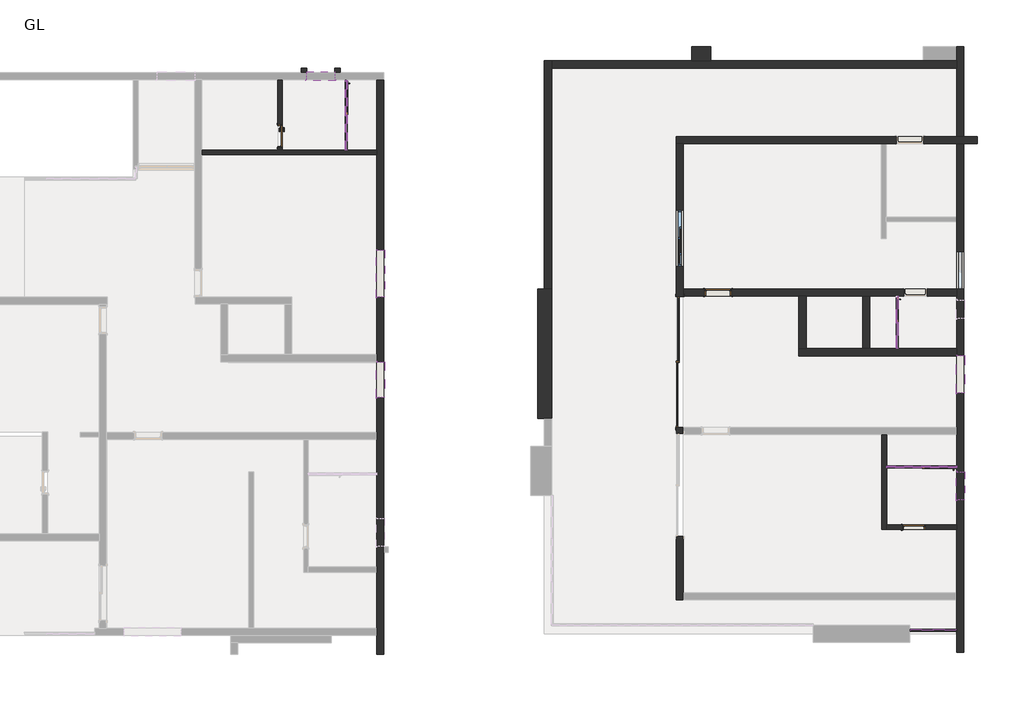
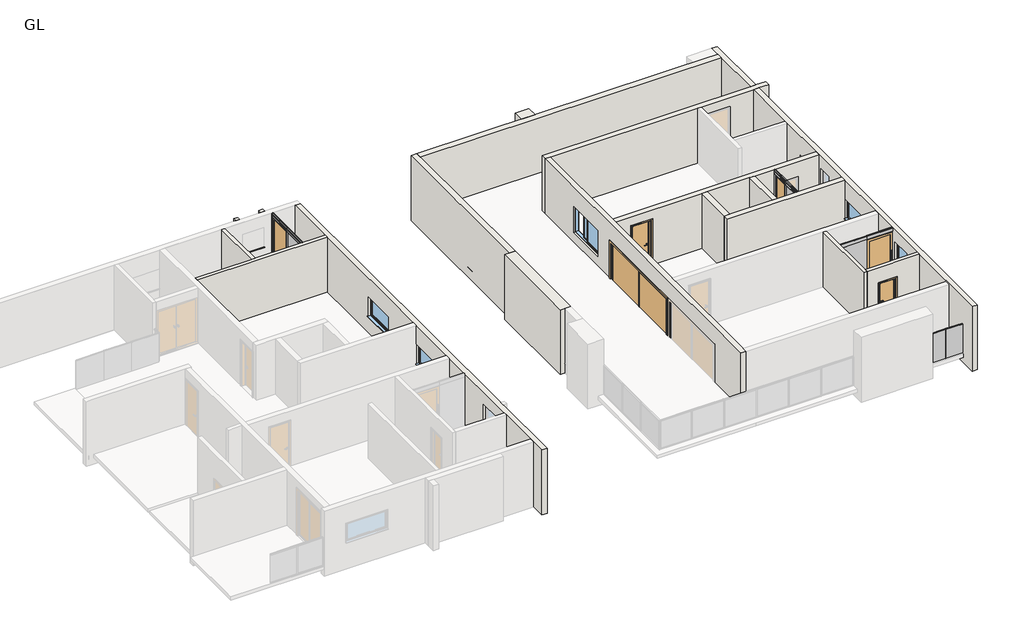
# One storey, part 4 of 6: 41 members, 18 walls, 11 plates, 7 doors, 6 windows.
"""IFC4 building model written with IfcOpenShell, lengths in millimetres."""

from ifc_helpers import new_model, si_unit, frame, origin, origin_with_axes, place, context, project, spatial, polyline, outline, extrude, faceted_brep, transform, mapped, element, save
from components import door_14_4c4e9c4f, door_b7cddb0a, doors_intsgl_2_5_fba66aca, doors_sgl_glass_1_glass_panel_12mm_thickness_3d57b09a, doors_sgl_glass_1_glass_panel_12mm_thickness_ae7dd786, doors_sgl_glass_1_glass_panel_12mm_thickness_d76e1df9, rectangular_mullion_30mm_square_7ad516a4, rectangular_mullion_30mm_square_4b249e81, rectangular_mullion_30mm_square_9902f449, rectangular_mullion_30mm_square_eec092c3, rectangular_mullion_30mm_square_9325025b, rectangular_mullion_30mm_square_b25d63a0, rectangular_mullion_30mm_square_e994106c, rectangular_mullion_30mm_square_28ebc8b3, rectangular_mullion_30mm_square_b4ecd99e, rectangular_mullion_30mm_square_e2360202, rectangular_mullion_30mm_square_9211323b, rectangular_mullion_30mm_square_b0565101, rectangular_mullion_30mm_square_fdabec93, system_panel_glazed_78f80fad, system_panel_glazed_cac99656, system_panel_glazed_6c2d91e7, system_panel_glazed_d770e50e, system_panel_glazed_325d72d1, system_panel_glazed_2af15f36, system_panel_glazed_747750e0, parametric_operable_sliding_window_6387_6_8dd7d652, windows_sgl_plain_3_28d0678b, window_6a333e19, windows_sgl_plain_4_aaf4c78a, windows_sgl_plain_5_79f17ecf

model = new_model("IFC4")

# Units and contexts
model_context = context("Model", 3, world=origin())
ifc_project = project(units=[si_unit("LENGTHUNIT", "METRE", prefix="MILLI")], contexts=[model_context])

# Site, building, storey
site = spatial("IfcSite", under=ifc_project)
building = spatial("IfcBuilding", under=site)
storey = spatial("IfcBuildingStorey", under=building, Name="GL", Elevation=0.0)

# Doors
placement = place(None, origin())
door_14_shape = door_14_4c4e9c4f(model_context)
element("IfcDoor", 1, ObjectType="14'", at=placement, inside=storey, context=model_context, shape_type="MappedRepresentation", body=[
    mapped(door_14_shape, transform((-5795.6337573, 17869.1220058, 0.0), x_axis=(0.0, 1.0, 0.0), y_axis=(-1.0, 0.0, 0.0), z_axis=(0.0, 0.0, 1.0))),
])
door_shape = door_b7cddb0a(model_context)
element("IfcDoor", 2, ObjectType="Doors_IntSgl : 2'11\"", at=placement, inside=storey, context=model_context, shape_type="MappedRepresentation", body=[
    mapped(door_shape, transform((-4678.0337573, 20128.7664182, 449.9570313), x_axis=(-1.0, 0.0, 0.0), y_axis=(0.0, -1.0, 0.0), z_axis=(0.0, 0.0, 1.0))),
])
doors_intsgl_2_5_shape = doors_intsgl_2_5_fba66aca(model_context)
element("IfcDoor", 3, ObjectType="Doors_IntSgl : 2.5'", at=placement, inside=storey, context=model_context, shape_type="MappedRepresentation", body=[
    mapped(doors_intsgl_2_5_shape, transform((-18933.3266085, 25228.098106, 0.0), x_axis=(0.0, -1.0, 0.0), y_axis=(1.0, 0.0, 0.0), z_axis=(0.0, 0.0, 1.0))),
])
element("IfcDoor", 4, ObjectType="Doors_IntSgl : 2.5'", at=placement, inside=storey, context=model_context, shape_type="MappedRepresentation", body=[
    mapped(doors_intsgl_2_5_shape, transform((1696.7626485, 12484.3220058, 449.9570313), x_axis=(1.0, 0.0, 0.0), y_axis=(0.0, 1.0, 0.0), z_axis=(0.0, 0.0, 1.0))),
])
doors_sgl_glass_1_glass_panel_12mm_thickness_shape = doors_sgl_glass_1_glass_panel_12mm_thickness_3d57b09a(model_context)
element("IfcDoor", 5, ObjectType="Doors_Sgl_Glass_1 : Glass_Panel-12mm_Thickness", at=placement, inside=storey, context=model_context, shape_type="MappedRepresentation", body=[
    mapped(doors_sgl_glass_1_glass_panel_12mm_thickness_shape, transform((-16799.7266085, 26469.8075628, 479.9570313), x_axis=(0.0, -1.0, 0.0), y_axis=(1.0, 0.0, 0.0), z_axis=(0.0, 0.0, 1.0))),
])
doors_sgl_glass_1_glass_panel_12mm_thickness_2_shape = doors_sgl_glass_1_glass_panel_12mm_thickness_ae7dd786(model_context)
element("IfcDoor", 6, ObjectType="Doors_Sgl_Glass_1 : Glass_Panel-12mm_Thickness", at=placement, inside=storey, context=model_context, shape_type="MappedRepresentation", body=[
    mapped(doors_sgl_glass_1_glass_panel_12mm_thickness_2_shape, transform((2515.5764369, 14465.5220058, 479.9570313), x_axis=(-1.0, 0.0, 0.0), y_axis=(0.0, -1.0, 0.0), z_axis=(0.0, 0.0, 1.0))),
])
doors_sgl_glass_1_glass_panel_12mm_thickness_3_shape = doors_sgl_glass_1_glass_panel_12mm_thickness_d76e1df9(model_context)
element("IfcDoor", 7, ObjectType="Doors_Sgl_Glass_1 : Glass_Panel-12mm_Thickness", at=placement, inside=storey, context=model_context, shape_type="MappedRepresentation", body=[
    mapped(doors_sgl_glass_1_glass_panel_12mm_thickness_3_shape, transform((1132.6976997, 19578.0085204, 479.9570313), x_axis=(0.0, -1.0, 0.0), y_axis=(1.0, 0.0, 0.0), z_axis=(0.0, 0.0, 1.0))),
])

# Members
rectangular_mullion_30mm_square_shape = rectangular_mullion_30mm_square_7ad516a4(model_context)
element("IfcMember", 8, ObjectType="Rectangular Mullion : 30mm_Square", at=placement, inside=storey, context=model_context, shape_type="MappedRepresentation", body=[
    mapped(rectangular_mullion_30mm_square_shape, transform((2330.3942124, 9140.7448884, 449.9570313), x_axis=(-1.0, 0.0, 0.0), y_axis=(0.0, 1.0, 0.0), z_axis=(0.0, 0.0, -1.0))),
])
rectangular_mullion_30mm_square_2_shape = rectangular_mullion_30mm_square_4b249e81(model_context)
element("IfcMember", 9, ObjectType="Rectangular Mullion : 30mm_Square", at=placement, inside=storey, context=model_context, shape_type="MappedRepresentation", body=[
    mapped(rectangular_mullion_30mm_square_2_shape, transform((3094.8476997, 9140.7448884, 1780.8), x_axis=(1.0, 0.0, 0.0), y_axis=(0.0, 1.0, 0.0), z_axis=(0.0, 0.0, 1.0))),
])
element("IfcMember", 10, ObjectType="Rectangular Mullion : 30mm_Square", at=placement, inside=storey, context=model_context, shape_type="MappedRepresentation", body=[
    mapped(rectangular_mullion_30mm_square_2_shape, transform((1565.9407251, 9140.7448884, 449.9570313), x_axis=(-1.0, 0.0, 0.0), y_axis=(0.0, 1.0, 0.0), z_axis=(0.0, 0.0, -1.0))),
])
rectangular_mullion_30mm_square_3_shape = rectangular_mullion_30mm_square_9902f449(model_context)
element("IfcMember", 11, ObjectType="Rectangular Mullion : 30mm_Square", at=placement, inside=storey, context=model_context, shape_type="MappedRepresentation", body=[
    mapped(rectangular_mullion_30mm_square_3_shape, transform((1595.9407251, 9140.7448884, 1780.8), x_axis=(0.0, 0.0, 1.0), y_axis=(0.0, 1.0, 0.0), z_axis=(-1.0, 0.0, 0.0))),
])
element("IfcMember", 12, ObjectType="Rectangular Mullion : 30mm_Square", at=placement, inside=storey, context=model_context, shape_type="MappedRepresentation", body=[
    mapped(rectangular_mullion_30mm_square_3_shape, transform((2345.3942124, 9140.7448884, 1780.8), x_axis=(0.0, 0.0, 1.0), y_axis=(0.0, 1.0, 0.0), z_axis=(-1.0, 0.0, 0.0))),
])
element("IfcMember", 13, ObjectType="Rectangular Mullion : 30mm_Square", at=placement, inside=storey, context=model_context, shape_type="MappedRepresentation", body=[
    mapped(rectangular_mullion_30mm_square_3_shape, transform((3064.8476997, 9140.7448884, 449.9570313), x_axis=(0.0, 0.0, -1.0), y_axis=(0.0, 1.0, 0.0), z_axis=(1.0, 0.0, 0.0))),
])
element("IfcMember", 14, ObjectType="Rectangular Mullion : 30mm_Square", at=placement, inside=storey, context=model_context, shape_type="MappedRepresentation", body=[
    mapped(rectangular_mullion_30mm_square_3_shape, transform((2315.3942124, 9140.7448884, 449.9570313), x_axis=(0.0, 0.0, -1.0), y_axis=(0.0, 1.0, 0.0), z_axis=(1.0, 0.0, 0.0))),
])
rectangular_mullion_30mm_square_4_shape = rectangular_mullion_30mm_square_eec092c3(model_context)
element("IfcMember", 15, ObjectType="Rectangular Mullion : 30mm_Square", at=placement, inside=storey, context=model_context, shape_type="MappedRepresentation", body=[
    mapped(rectangular_mullion_30mm_square_4_shape, transform((-16799.7266085, 24800.898106, 3000.0), x_axis=(0.0, 0.0, 1.0), y_axis=(-1.0, 0.0, 0.0), z_axis=(0.0, -1.0, 0.0))),
])
element("IfcMember", 16, ObjectType="Rectangular Mullion : 30mm_Square", at=placement, inside=storey, context=model_context, shape_type="MappedRepresentation", body=[
    mapped(rectangular_mullion_30mm_square_4_shape, transform((-16799.7266085, 25923.5044105, 3000.0), x_axis=(0.0, 0.0, 1.0), y_axis=(-1.0, 0.0, 0.0), z_axis=(0.0, -1.0, 0.0))),
])
element("IfcMember", 17, ObjectType="Rectangular Mullion : 30mm_Square", at=placement, inside=storey, context=model_context, shape_type="MappedRepresentation", body=[
    mapped(rectangular_mullion_30mm_square_4_shape, transform((-16799.7266085, 27016.1107151, 449.9570313), x_axis=(0.0, 0.0, -1.0), y_axis=(-1.0, 0.0, 0.0), z_axis=(0.0, 1.0, 0.0))),
])
element("IfcMember", 18, ObjectType="Rectangular Mullion : 30mm_Square", at=placement, inside=storey, context=model_context, shape_type="MappedRepresentation", body=[
    mapped(rectangular_mullion_30mm_square_4_shape, transform((-16799.7266085, 25893.5044105, 449.9570313), x_axis=(0.0, 0.0, -1.0), y_axis=(-1.0, 0.0, 0.0), z_axis=(0.0, 1.0, 0.0))),
])
rectangular_mullion_30mm_square_5_shape = rectangular_mullion_30mm_square_9325025b(model_context)
element("IfcMember", 19, ObjectType="Rectangular Mullion : 30mm_Square", at=placement, inside=storey, context=model_context, shape_type="MappedRepresentation", body=[
    mapped(rectangular_mullion_30mm_square_5_shape, transform((-16799.7266085, 25908.5044105, 449.9570313), x_axis=(0.0, -1.0, 0.0), y_axis=(-1.0, 0.0, 0.0), z_axis=(0.0, 0.0, -1.0))),
])
element("IfcMember", 20, ObjectType="Rectangular Mullion : 30mm_Square", at=placement, inside=storey, context=model_context, shape_type="MappedRepresentation", body=[
    mapped(rectangular_mullion_30mm_square_5_shape, transform((1951.3051741, 14465.5220058, 449.9570313), x_axis=(-1.0, 0.0, 0.0), y_axis=(0.0, 1.0, 0.0), z_axis=(0.0, 0.0, -1.0))),
])
element("IfcMember", 21, ObjectType="Rectangular Mullion : 30mm_Square", at=placement, inside=storey, context=model_context, shape_type="MappedRepresentation", body=[
    mapped(rectangular_mullion_30mm_square_5_shape, transform((1132.6976997, 19156.5506226, 449.9570313), x_axis=(0.0, -1.0, 0.0), y_axis=(-1.0, 0.0, 0.0), z_axis=(0.0, 0.0, -1.0))),
])
rectangular_mullion_30mm_square_6_shape = rectangular_mullion_30mm_square_b25d63a0(model_context)
element("IfcMember", 22, ObjectType="Rectangular Mullion : 30mm_Square", at=placement, inside=storey, context=model_context, shape_type="MappedRepresentation", body=[
    mapped(rectangular_mullion_30mm_square_6_shape, transform((-16799.7266085, 25923.5044105, 2849.9570312), x_axis=(0.0, 0.0, 1.0), y_axis=(-1.0, 0.0, 0.0), z_axis=(0.0, -1.0, 0.0))),
])
element("IfcMember", 23, ObjectType="Rectangular Mullion : 30mm_Square", at=placement, inside=storey, context=model_context, shape_type="MappedRepresentation", body=[
    mapped(rectangular_mullion_30mm_square_6_shape, transform((-16799.7266085, 24800.898106, 2849.9570312), x_axis=(0.0, 0.0, 1.0), y_axis=(-1.0, 0.0, 0.0), z_axis=(0.0, -1.0, 0.0))),
])
rectangular_mullion_30mm_square_7_shape = rectangular_mullion_30mm_square_e994106c(model_context)
element("IfcMember", 24, ObjectType="Rectangular Mullion : 30mm_Square", at=placement, inside=storey, context=model_context, shape_type="MappedRepresentation", body=[
    mapped(rectangular_mullion_30mm_square_7_shape, transform((-16799.7266085, 25908.5044105, 2849.9570312), x_axis=(0.0, -1.0, 0.0), y_axis=(-1.0, 0.0, 0.0), z_axis=(0.0, 0.0, -1.0))),
])
element("IfcMember", 25, ObjectType="Rectangular Mullion : 30mm_Square", at=placement, inside=storey, context=model_context, shape_type="MappedRepresentation", body=[
    mapped(rectangular_mullion_30mm_square_7_shape, transform((1951.3051741, 14465.5220058, 2849.9570312), x_axis=(-1.0, 0.0, 0.0), y_axis=(0.0, 1.0, 0.0), z_axis=(0.0, 0.0, -1.0))),
])
element("IfcMember", 26, ObjectType="Rectangular Mullion : 30mm_Square", at=placement, inside=storey, context=model_context, shape_type="MappedRepresentation", body=[
    mapped(rectangular_mullion_30mm_square_7_shape, transform((1132.6976997, 19156.5506226, 2849.9570312), x_axis=(0.0, -1.0, 0.0), y_axis=(-1.0, 0.0, 0.0), z_axis=(0.0, 0.0, -1.0))),
])
rectangular_mullion_30mm_square_8_shape = rectangular_mullion_30mm_square_28ebc8b3(model_context)
element("IfcMember", 27, ObjectType="Rectangular Mullion : 30mm_Square", at=placement, inside=storey, context=model_context, shape_type="MappedRepresentation", body=[
    mapped(rectangular_mullion_30mm_square_8_shape, transform((-16799.7266085, 27046.1107151, 3000.0), x_axis=(0.0, 1.0, 0.0), y_axis=(-1.0, 0.0, 0.0), z_axis=(0.0, 0.0, 1.0))),
])
element("IfcMember", 28, ObjectType="Rectangular Mullion : 30mm_Square", at=placement, inside=storey, context=model_context, shape_type="MappedRepresentation", body=[
    mapped(rectangular_mullion_30mm_square_8_shape, transform((3094.8476997, 14465.5220058, 3000.0), x_axis=(1.0, 0.0, 0.0), y_axis=(0.0, 1.0, 0.0), z_axis=(0.0, 0.0, 1.0))),
])
rectangular_mullion_30mm_square_9_shape = rectangular_mullion_30mm_square_b4ecd99e(model_context)
element("IfcMember", 29, ObjectType="Rectangular Mullion : 30mm_Square", at=placement, inside=storey, context=model_context, shape_type="MappedRepresentation", body=[
    mapped(rectangular_mullion_30mm_square_9_shape, transform((-16799.7266085, 24770.898106, 449.9570313), x_axis=(0.0, -1.0, 0.0), y_axis=(-1.0, 0.0, 0.0), z_axis=(0.0, 0.0, -1.0))),
])
element("IfcMember", 30, ObjectType="Rectangular Mullion : 30mm_Square", at=placement, inside=storey, context=model_context, shape_type="MappedRepresentation", body=[
    mapped(rectangular_mullion_30mm_square_9_shape, transform((807.7626485, 14465.5220058, 449.9570313), x_axis=(-1.0, 0.0, 0.0), y_axis=(0.0, 1.0, 0.0), z_axis=(0.0, 0.0, -1.0))),
])
element("IfcMember", 31, ObjectType="Rectangular Mullion : 30mm_Square", at=placement, inside=storey, context=model_context, shape_type="MappedRepresentation", body=[
    mapped(rectangular_mullion_30mm_square_9_shape, transform((1132.6976997, 18298.634827, 449.9570313), x_axis=(0.0, -1.0, 0.0), y_axis=(-1.0, 0.0, 0.0), z_axis=(0.0, 0.0, -1.0))),
])
element("IfcMember", 32, ObjectType="Rectangular Mullion : 30mm_Square", at=placement, inside=storey, context=model_context, shape_type="MappedRepresentation", body=[
    mapped(rectangular_mullion_30mm_square_8_shape, transform((-16799.7266085, 24770.898106, 2849.9570312), x_axis=(0.0, -1.0, 0.0), y_axis=(-1.0, 0.0, 0.0), z_axis=(0.0, 0.0, -1.0))),
])
element("IfcMember", 33, ObjectType="Rectangular Mullion : 30mm_Square", at=placement, inside=storey, context=model_context, shape_type="MappedRepresentation", body=[
    mapped(rectangular_mullion_30mm_square_8_shape, transform((807.7626485, 14465.5220058, 2849.9570312), x_axis=(-1.0, 0.0, 0.0), y_axis=(0.0, 1.0, 0.0), z_axis=(0.0, 0.0, -1.0))),
])
element("IfcMember", 34, ObjectType="Rectangular Mullion : 30mm_Square", at=placement, inside=storey, context=model_context, shape_type="MappedRepresentation", body=[
    mapped(rectangular_mullion_30mm_square_8_shape, transform((1132.6976997, 18298.634827, 2849.9570312), x_axis=(0.0, -1.0, 0.0), y_axis=(-1.0, 0.0, 0.0), z_axis=(0.0, 0.0, -1.0))),
])
element("IfcMember", 35, ObjectType="Rectangular Mullion : 30mm_Square", at=placement, inside=storey, context=model_context, shape_type="MappedRepresentation", body=[
    mapped(rectangular_mullion_30mm_square_9_shape, transform((-16799.7266085, 27046.1107151, 2849.9570312), x_axis=(0.0, 1.0, 0.0), y_axis=(-1.0, 0.0, 0.0), z_axis=(0.0, 0.0, 1.0))),
])
element("IfcMember", 36, ObjectType="Rectangular Mullion : 30mm_Square", at=placement, inside=storey, context=model_context, shape_type="MappedRepresentation", body=[
    mapped(rectangular_mullion_30mm_square_9_shape, transform((3094.8476997, 14465.5220058, 2849.9570312), x_axis=(1.0, 0.0, 0.0), y_axis=(0.0, 1.0, 0.0), z_axis=(0.0, 0.0, 1.0))),
])
rectangular_mullion_30mm_square_10_shape = rectangular_mullion_30mm_square_e2360202(model_context)
element("IfcMember", 37, ObjectType="Rectangular Mullion : 30mm_Square", at=placement, inside=storey, context=model_context, shape_type="MappedRepresentation", body=[
    mapped(rectangular_mullion_30mm_square_10_shape, transform((837.7626485, 14465.5220058, 3000.0), x_axis=(0.0, 0.0, 1.0), y_axis=(0.0, 1.0, 0.0), z_axis=(-1.0, 0.0, 0.0))),
])
element("IfcMember", 38, ObjectType="Rectangular Mullion : 30mm_Square", at=placement, inside=storey, context=model_context, shape_type="MappedRepresentation", body=[
    mapped(rectangular_mullion_30mm_square_10_shape, transform((1966.3051741, 14465.5220058, 3000.0), x_axis=(0.0, 0.0, 1.0), y_axis=(0.0, 1.0, 0.0), z_axis=(-1.0, 0.0, 0.0))),
])
element("IfcMember", 39, ObjectType="Rectangular Mullion : 30mm_Square", at=placement, inside=storey, context=model_context, shape_type="MappedRepresentation", body=[
    mapped(rectangular_mullion_30mm_square_10_shape, transform((3064.8476997, 14465.5220058, 449.9570313), x_axis=(0.0, 0.0, -1.0), y_axis=(0.0, 1.0, 0.0), z_axis=(1.0, 0.0, 0.0))),
])
element("IfcMember", 40, ObjectType="Rectangular Mullion : 30mm_Square", at=placement, inside=storey, context=model_context, shape_type="MappedRepresentation", body=[
    mapped(rectangular_mullion_30mm_square_10_shape, transform((1936.3051741, 14465.5220058, 449.9570313), x_axis=(0.0, 0.0, -1.0), y_axis=(0.0, 1.0, 0.0), z_axis=(1.0, 0.0, 0.0))),
])
rectangular_mullion_30mm_square_11_shape = rectangular_mullion_30mm_square_9211323b(model_context)
element("IfcMember", 41, ObjectType="Rectangular Mullion : 30mm_Square", at=placement, inside=storey, context=model_context, shape_type="MappedRepresentation", body=[
    mapped(rectangular_mullion_30mm_square_11_shape, transform((1966.3051741, 14465.5220058, 2849.9570312), x_axis=(0.0, 0.0, 1.0), y_axis=(0.0, 1.0, 0.0), z_axis=(-1.0, 0.0, 0.0))),
])
element("IfcMember", 42, ObjectType="Rectangular Mullion : 30mm_Square", at=placement, inside=storey, context=model_context, shape_type="MappedRepresentation", body=[
    mapped(rectangular_mullion_30mm_square_11_shape, transform((837.7626485, 14465.5220058, 2849.9570312), x_axis=(0.0, 0.0, 1.0), y_axis=(0.0, 1.0, 0.0), z_axis=(-1.0, 0.0, 0.0))),
])
rectangular_mullion_30mm_square_12_shape = rectangular_mullion_30mm_square_b0565101(model_context)
element("IfcMember", 43, ObjectType="Rectangular Mullion : 30mm_Square", at=placement, inside=storey, context=model_context, shape_type="MappedRepresentation", body=[
    mapped(rectangular_mullion_30mm_square_12_shape, transform((1132.6976997, 18328.634827, 3000.0), x_axis=(0.0, 0.0, 1.0), y_axis=(-1.0, 0.0, 0.0), z_axis=(0.0, -1.0, 0.0))),
])
element("IfcMember", 44, ObjectType="Rectangular Mullion : 30mm_Square", at=placement, inside=storey, context=model_context, shape_type="MappedRepresentation", body=[
    mapped(rectangular_mullion_30mm_square_12_shape, transform((1132.6976997, 19171.5506226, 3000.0), x_axis=(0.0, 0.0, 1.0), y_axis=(-1.0, 0.0, 0.0), z_axis=(0.0, -1.0, 0.0))),
])
element("IfcMember", 45, ObjectType="Rectangular Mullion : 30mm_Square", at=placement, inside=storey, context=model_context, shape_type="MappedRepresentation", body=[
    mapped(rectangular_mullion_30mm_square_12_shape, transform((1132.6976997, 19984.4664182, 449.9570313), x_axis=(0.0, 0.0, -1.0), y_axis=(-1.0, 0.0, 0.0), z_axis=(0.0, 1.0, 0.0))),
])
element("IfcMember", 46, ObjectType="Rectangular Mullion : 30mm_Square", at=placement, inside=storey, context=model_context, shape_type="MappedRepresentation", body=[
    mapped(rectangular_mullion_30mm_square_12_shape, transform((1132.6976997, 19141.5506226, 449.9570313), x_axis=(0.0, 0.0, -1.0), y_axis=(-1.0, 0.0, 0.0), z_axis=(0.0, 1.0, 0.0))),
])
rectangular_mullion_30mm_square_13_shape = rectangular_mullion_30mm_square_fdabec93(model_context)
element("IfcMember", 47, ObjectType="Rectangular Mullion : 30mm_Square", at=placement, inside=storey, context=model_context, shape_type="MappedRepresentation", body=[
    mapped(rectangular_mullion_30mm_square_13_shape, transform((1132.6976997, 19171.5506226, 2849.9570312), x_axis=(0.0, 0.0, 1.0), y_axis=(-1.0, 0.0, 0.0), z_axis=(0.0, -1.0, 0.0))),
])
element("IfcMember", 48, ObjectType="Rectangular Mullion : 30mm_Square", at=placement, inside=storey, context=model_context, shape_type="MappedRepresentation", body=[
    mapped(rectangular_mullion_30mm_square_13_shape, transform((1132.6976997, 18328.634827, 2849.9570312), x_axis=(0.0, 0.0, 1.0), y_axis=(-1.0, 0.0, 0.0), z_axis=(0.0, -1.0, 0.0))),
])

# Plates
system_panel_glazed_shape = system_panel_glazed_78f80fad(model_context)
element("IfcPlate", 49, ObjectType="System Panel : Glazed", at=placement, inside=storey, context=model_context, shape_type="MappedRepresentation", body=[
    mapped(system_panel_glazed_shape, transform((2712.6209561, 9140.7448884, 449.9570313), x_axis=(-1.0, 0.0, 0.0), y_axis=(0.0, -1.0, 0.0), z_axis=(0.0, 0.0, 1.0))),
])
element("IfcPlate", 50, ObjectType="System Panel : Glazed", at=placement, inside=storey, context=model_context, shape_type="MappedRepresentation", body=[
    mapped(system_panel_glazed_shape, transform((1948.1674688, 9140.7448884, 449.9570313), x_axis=(-1.0, 0.0, 0.0), y_axis=(0.0, -1.0, 0.0), z_axis=(0.0, 0.0, 1.0))),
])
system_panel_glazed_2_shape = system_panel_glazed_cac99656(model_context)
element("IfcPlate", 51, ObjectType="System Panel : Glazed", at=placement, inside=storey, context=model_context, shape_type="MappedRepresentation", body=[
    mapped(system_panel_glazed_2_shape, transform((-16799.7266085, 25339.7012583, 449.9570313), x_axis=(0.0, -1.0, 0.0), y_axis=(1.0, 0.0, 0.0), z_axis=(0.0, 0.0, 1.0))),
])
system_panel_glazed_3_shape = system_panel_glazed_6c2d91e7(model_context)
element("IfcPlate", 52, ObjectType="System Panel : Glazed", at=placement, inside=storey, context=model_context, shape_type="MappedRepresentation", body=[
    mapped(system_panel_glazed_3_shape, transform((-16799.7266085, 26477.3075628, 2849.9570312), x_axis=(0.0, -1.0, 0.0), y_axis=(1.0, 0.0, 0.0), z_axis=(0.0, 0.0, 1.0))),
])
element("IfcPlate", 53, ObjectType="System Panel : Glazed", at=placement, inside=storey, context=model_context, shape_type="MappedRepresentation", body=[
    mapped(system_panel_glazed_3_shape, transform((-16799.7266085, 25339.7012583, 2849.9570312), x_axis=(0.0, -1.0, 0.0), y_axis=(1.0, 0.0, 0.0), z_axis=(0.0, 0.0, 1.0))),
])
system_panel_glazed_4_shape = system_panel_glazed_d770e50e(model_context)
element("IfcPlate", 54, ObjectType="System Panel : Glazed", at=placement, inside=storey, context=model_context, shape_type="MappedRepresentation", body=[
    mapped(system_panel_glazed_4_shape, transform((1379.5339113, 14465.5220058, 449.9570313), x_axis=(-1.0, 0.0, 0.0), y_axis=(0.0, -1.0, 0.0), z_axis=(0.0, 0.0, 1.0))),
])
system_panel_glazed_5_shape = system_panel_glazed_325d72d1(model_context)
element("IfcPlate", 55, ObjectType="System Panel : Glazed", at=placement, inside=storey, context=model_context, shape_type="MappedRepresentation", body=[
    mapped(system_panel_glazed_5_shape, transform((2523.0764369, 14465.5220058, 2849.9570312), x_axis=(-1.0, 0.0, 0.0), y_axis=(0.0, -1.0, 0.0), z_axis=(0.0, 0.0, 1.0))),
])
element("IfcPlate", 56, ObjectType="System Panel : Glazed", at=placement, inside=storey, context=model_context, shape_type="MappedRepresentation", body=[
    mapped(system_panel_glazed_5_shape, transform((1379.5339113, 14465.5220058, 2849.9570312), x_axis=(-1.0, 0.0, 0.0), y_axis=(0.0, -1.0, 0.0), z_axis=(0.0, 0.0, 1.0))),
])
system_panel_glazed_6_shape = system_panel_glazed_2af15f36(model_context)
element("IfcPlate", 57, ObjectType="System Panel : Glazed", at=placement, inside=storey, context=model_context, shape_type="MappedRepresentation", body=[
    mapped(system_panel_glazed_6_shape, transform((1132.6976997, 18727.5927248, 449.9570313), x_axis=(0.0, -1.0, 0.0), y_axis=(1.0, 0.0, 0.0), z_axis=(0.0, 0.0, 1.0))),
])
system_panel_glazed_7_shape = system_panel_glazed_747750e0(model_context)
element("IfcPlate", 58, ObjectType="System Panel : Glazed", at=placement, inside=storey, context=model_context, shape_type="MappedRepresentation", body=[
    mapped(system_panel_glazed_7_shape, transform((1132.6976997, 19585.5085204, 2849.9570312), x_axis=(0.0, -1.0, 0.0), y_axis=(1.0, 0.0, 0.0), z_axis=(0.0, 0.0, 1.0))),
])
element("IfcPlate", 59, ObjectType="System Panel : Glazed", at=placement, inside=storey, context=model_context, shape_type="MappedRepresentation", body=[
    mapped(system_panel_glazed_7_shape, transform((1132.6976997, 18727.5927248, 2849.9570312), x_axis=(0.0, -1.0, 0.0), y_axis=(1.0, 0.0, 0.0), z_axis=(0.0, 0.0, 1.0))),
])

# Walls
element("IfcWall", 60, ObjectType="1'6\"", at=placement, inside=storey, context=model_context, shape_type="Brep", body=[
    faceted_brep([(-10088.6061453, 16028.5795779, 0.0), (-10088.6061453, 20244.9795779, 0.0), (-10088.6061453, 20244.9795779, 3000.0), (-10088.6061453, 16028.5795779, 3000.0), (-10545.8061453, 16028.5795779, 0.0), (-10545.8061453, 16028.5795779, 3000.0), (-10545.8061453, 20244.9795779, 3000.0), (-10545.8061453, 20244.9795779, 0.0), (-10342.6061453, 16028.5795779, 0.0), (-10342.6061453, 20244.9795779, 0.0), (-10342.6061453, 20244.9795779, 3000.0), (-10342.6061453, 16028.5795779, 3000.0)], [[[0, 1, 2, 3]], [[4, 5, 6, 7]], [[1, 0, 8, 4, 7, 9]], [[2, 1, 9, 7, 6, 10]], [[3, 2, 10, 6, 5, 11]], [[0, 3, 11, 5, 4, 8]]]),
])
element("IfcWall", 61, ObjectType="1'6\"", at=placement, inside=storey, context=model_context, shape_type="SweptSolid", body=[
    extrude(outline(polyline([(-4916.7705321, 27687.1795779), (-5526.3705321, 27687.1795779), (-5526.3705321, 28144.3795779), (-4916.7705321, 28144.3795779), (-4916.7705321, 27687.1795779)])), origin_with_axes(), (0.0, 0.0, 1.0), 3000.0),
])
element("IfcWall", 62, ObjectType="10\"", at=placement, inside=storey, context=model_context, shape_type="Brep", body=[
    faceted_brep([(-10088.6061453, 20244.9795779, 0.0), (-10088.6061453, 27433.1795779, 0.0), (-10088.6061453, 27687.1795779, 0.0), (-10088.6061453, 27687.1795779, 3000.0), (-10088.6061453, 27433.1795779, 3000.0), (-10088.6061453, 20244.9795779, 3000.0), (-10342.6061453, 20244.9795779, 0.0), (-10342.6061453, 20244.9795779, 3000.0), (-10342.6061453, 27687.1795779, 3000.0), (-10342.6061453, 27687.1795779, 0.0)], [[[0, 1, 2, 3, 4, 5]], [[6, 7, 8, 9]], [[2, 1, 0, 6, 9]], [[5, 4, 3, 8, 7]], [[0, 5, 7, 6]], [[3, 2, 9, 8]]]),
])
element("IfcWall", 63, ObjectType="10\"", at=placement, inside=storey, context=model_context, shape_type="SweptSolid", body=[
    extrude(outline(polyline([(3094.8476997, 27433.1795779), (-10088.6061453, 27433.1795779), (-10088.6061453, 27687.1795779), (3094.8476997, 27687.1795779), (3094.8476997, 27433.1795779)])), origin_with_axes(), (0.0, 0.0, 1.0), 3000.0),
])
element("IfcWall", 64, ObjectType="6\" WALL", at=placement, inside=storey, context=model_context, shape_type="Brep", body=[
    faceted_brep([(-15785.4464918, 24770.898106, 0.0), (-18857.1266085, 24770.898106, 0.0), (-19009.5266085, 24770.898106, 0.0), (-21486.3263661, 24770.898106, 0.0), (-21486.3263661, 24770.898106, 3000.0), (-19009.5266085, 24770.898106, 3000.0), (-18857.1266085, 24770.898106, 3000.0), (-15785.4464918, 24770.898106, 3000.0), (-15785.4464918, 24618.498106, 0.0), (-15785.4464918, 24618.498106, 3000.0), (-21486.3263661, 24618.498106, 3000.0), (-21486.3263661, 24618.498106, 0.0)], [[[0, 1, 2, 3, 4, 5, 6, 7]], [[8, 9, 10, 11]], [[3, 2, 1, 0, 8, 11]], [[7, 6, 5, 4, 10, 9]], [[0, 7, 9, 8]], [[4, 3, 11, 10]]]),
])
element("IfcWall", 65, ObjectType="6\" WALL", at=placement, inside=storey, context=model_context, shape_type="SweptSolid", body=[
    extrude(outline(polyline([(24770.898106, 3000.0), (27056.898106, 3000.0), (27056.898106, 0.0), (25609.098106, 0.0), (25609.098106, 1828.8), (24847.098106, 1828.8), (24847.098106, 0.0), (24770.898106, 0.0), (24770.898106, 3000.0)])), frame((-19009.5266085, 0.0, 0.0), z_axis=(1.0, 0.0, 0.0), x_axis=(0.0, 1.0, 0.0)), (0.0, 0.0, 1.0), 152.4),
])
element("IfcWall", 66, ObjectType="6\" WALL", at=placement, inside=storey, context=model_context, shape_type="Brep", body=[
    faceted_brep([(655.3626485, 15506.9220058, 0.0), (655.3626485, 12408.1220058, 0.0), (655.3626485, 12408.1220058, 3000.0), (655.3626485, 15506.9220058, 3000.0), (807.7626485, 15506.9220058, 0.0), (807.7626485, 15506.9220058, 3000.0), (807.7626485, 12560.5220058, 3000.0), (807.7626485, 12408.1220058, 3000.0), (807.7626485, 12408.1220058, 0.0), (807.7626485, 12560.5220058, 0.0)], [[[0, 1, 2, 3]], [[4, 5, 6, 7, 8, 9]], [[1, 0, 4, 9, 8]], [[3, 2, 7, 6, 5]], [[0, 3, 5, 4]], [[2, 1, 8, 7]]]),
])
element("IfcWall", 67, ObjectType="6\" WALL", at=placement, inside=storey, context=model_context, shape_type="SweptSolid", body=[
    extrude(outline(polyline([(0.0, 3094.8476997), (3000.0, 3094.8476997), (3000.0, 807.7626485), (0.0, 807.7626485), (0.0, 3094.8476997)]), holes=[polyline([(449.9570313, 2077.7626485), (449.9570313, 1315.7626485), (2278.7570313, 1315.7626485), (2278.7570313, 2077.7626485), (449.9570313, 2077.7626485)])]), frame((0.0, 12408.1220058, 0.0), z_axis=(0.0, 1.0, 0.0), x_axis=(0.0, 0.0, 1.0)), (0.0, 0.0, 1.0), 152.4),
])
element("IfcWall", 68, ObjectType="7\" WALL", at=placement, inside=storey, context=model_context, shape_type="SweptSolid", body=[
    extrude(outline(polyline([(-18069.7266085, 27437.898106), (-18069.7266085, 27287.6409184), (-18247.5266085, 27287.6409184), (-18247.5266085, 27437.898106), (-18069.7266085, 27437.898106)])), origin_with_axes(), (0.0, 0.0, 1.0), 3000.0),
])
element("IfcWall", 69, ObjectType="7\" WALL", at=placement, inside=storey, context=model_context, shape_type="SweptSolid", body=[
    extrude(outline(polyline([(-16977.5266085, 27440.0409184), (-16977.5266085, 27287.6409184), (-17155.3266085, 27287.6409184), (-17155.3266085, 27440.0409184), (-16977.5266085, 27440.0409184)])), origin_with_axes(), (0.0, 0.0, 1.0), 3000.0),
])
element("IfcWall", 70, ObjectType="9\" INNER WALL", at=placement, inside=storey, context=model_context, shape_type="Brep", body=[
    faceted_brep([(-15556.8464918, 8339.2409184, 0.0), (-15556.8464918, 11672.6322323, 0.0), (-15556.8464918, 11850.4322323, 0.0), (-15556.8464918, 27059.0409184, 0.0), (-15556.8464918, 27059.0409184, 3000.0), (-15556.8464918, 11850.4322323, 3000.0), (-15556.8464918, 11672.6322323, 3000.0), (-15556.8464918, 8339.2409184, 3000.0), (-15556.8464918, 21506.998106, 2110.0), (-15556.8464918, 21506.998106, 1200.0), (-15556.8464918, 19982.998106, 1200.0), (-15556.8464918, 19982.998106, 2110.0), (-15556.8464918, 17874.798106, 2110.0), (-15556.8464918, 17874.798106, 1200.0), (-15556.8464918, 16706.398106, 1200.0), (-15556.8464918, 16706.398106, 2110.0), (-15556.8464918, 12771.1822323, 2434.0), (-15556.8464918, 12771.1822323, 1524.0), (-15556.8464918, 11856.7822323, 1524.0), (-15556.8464918, 11856.7822323, 2434.0), (-15785.4464918, 8339.2409184, 0.0), (-15785.4464918, 8339.2409184, 3000.0), (-15785.4464918, 8962.7302878, 3000.0), (-15785.4464918, 9191.3302878, 3000.0), (-15785.4464918, 11018.5822323, 3000.0), (-15785.4464918, 11196.3822323, 3000.0), (-15785.4464918, 15349.2822323, 3000.0), (-15785.4464918, 15577.8822323, 3000.0), (-15785.4464918, 17874.798106, 3000.0), (-15785.4464918, 18103.398106, 3000.0), (-15785.4464918, 24618.498106, 3000.0), (-15785.4464918, 24770.898106, 3000.0), (-15785.4464918, 27059.0409184, 3000.0), (-15785.4464918, 27059.0409184, 0.0), (-15785.4464918, 24770.898106, 0.0), (-15785.4464918, 24618.498106, 0.0), (-15785.4464918, 18103.398106, 0.0), (-15785.4464918, 17874.798106, 0.0), (-15785.4464918, 15577.8822323, 0.0), (-15785.4464918, 15349.2822323, 0.0), (-15785.4464918, 11196.3822323, 0.0), (-15785.4464918, 11018.5822323, 0.0), (-15785.4464918, 9191.3302878, 0.0), (-15785.4464918, 8962.7302878, 0.0), (-15785.4464918, 21506.998106, 2110.0), (-15785.4464918, 19982.998106, 2110.0), (-15785.4464918, 19982.998106, 1200.0), (-15785.4464918, 21506.998106, 1200.0), (-15785.4464918, 17874.798106, 2110.0), (-15785.4464918, 16706.398106, 2110.0), (-15785.4464918, 16706.398106, 1200.0), (-15785.4464918, 17874.798106, 1200.0), (-15785.4464918, 12771.1822323, 2434.0), (-15785.4464918, 11856.7822323, 2434.0), (-15785.4464918, 11856.7822323, 1524.0), (-15785.4464918, 12771.1822323, 1524.0)], [[[0, 1, 2, 3, 4, 5, 6, 7], [8, 9, 10, 11], [12, 13, 14, 15], [16, 17, 18, 19]], [[20, 21, 22, 23, 24, 25, 26, 27, 28, 29, 30, 31, 32, 33, 34, 35, 36, 37, 38, 39, 40, 41, 42, 43], [44, 45, 46, 47], [48, 49, 50, 51], [52, 53, 54, 55]], [[3, 2, 1, 0, 20, 43, 42, 41, 40, 39, 38, 37, 36, 35, 34, 33]], [[7, 6, 5, 4, 32, 31, 30, 29, 28, 27, 26, 25, 24, 23, 22, 21]], [[0, 7, 21, 20]], [[4, 3, 33, 32]], [[9, 8, 44, 47]], [[10, 9, 47, 46]], [[11, 10, 46, 45]], [[8, 11, 45, 44]], [[13, 12, 48, 51]], [[14, 13, 51, 50]], [[15, 14, 50, 49]], [[12, 15, 49, 48]], [[17, 16, 52, 55]], [[18, 17, 55, 54]], [[19, 18, 54, 53]], [[16, 19, 53, 52]]]),
])
element("IfcWall", 71, ObjectType="9\" INNER WALL", at=placement, inside=storey, context=model_context, shape_type="Brep", body=[
    faceted_brep([(-6036.9337573, 24983.9592769, 0.0), (-5808.3337573, 24983.9592769, 0.0), (643.2662427, 24983.9592769, 0.0), (795.6662427, 24983.9592769, 0.0), (3094.8476997, 24983.9592769, 0.0), (3323.4476997, 24983.9592769, 0.0), (3767.4662427, 24983.9592769, 0.0), (3767.4662427, 24983.9592769, 3000.0), (3323.4476997, 24983.9592769, 3000.0), (3094.8476997, 24983.9592769, 3000.0), (795.6662427, 24983.9592769, 3000.0), (643.2662427, 24983.9592769, 3000.0), (-5808.3337573, 24983.9592769, 3000.0), (-6036.9337573, 24983.9592769, 3000.0), (2014.8662427, 24983.9592769, 2559.9570312), (2014.8662427, 24983.9592769, 449.9570313), (1125.8662427, 24983.9592769, 449.9570313), (1125.8662427, 24983.9592769, 2559.9570312), (3767.4662427, 25212.5592769, 0.0), (3323.4476997, 25212.5592769, 0.0), (3094.8476997, 25212.5592769, 0.0), (-6036.9337573, 25212.5592769, 0.0), (-6036.9337573, 25212.5592769, 3000.0), (3094.8476997, 25212.5592769, 3000.0), (3323.4476997, 25212.5592769, 3000.0), (3767.4662427, 25212.5592769, 3000.0), (2014.8662427, 25212.5592769, 449.9570313), (2014.8662427, 25212.5592769, 2559.9570312), (1125.8662427, 25212.5592769, 2559.9570312), (1125.8662427, 25212.5592769, 449.9570313)], [[[0, 1, 2, 3, 4, 5, 6, 7, 8, 9, 10, 11, 12, 13], [14, 15, 16, 17]], [[18, 19, 20, 21, 22, 23, 24, 25], [26, 27, 28, 29]], [[6, 5, 4, 3, 2, 1, 0, 21, 20, 19, 18]], [[7, 6, 18, 25]], [[13, 12, 11, 10, 9, 8, 7, 25, 24, 23, 22]], [[0, 13, 22, 21]], [[26, 15, 14, 27]], [[27, 14, 17, 28]], [[28, 17, 16, 29]], [[15, 26, 29, 16]]]),
])
element("IfcWall", 72, ObjectType="9\" INNER WALL", at=placement, inside=storey, context=model_context, shape_type="Brep", body=[
    faceted_brep([(-6036.9337573, 24983.9592769, 0.0), (-6036.9337573, 20002.7220058, 0.0), (-6036.9337573, 20002.7220058, 2134.0), (-6036.9337573, 15735.5220058, 2134.0), (-6036.9337573, 15735.5220058, 0.0), (-6036.9337573, 15535.1592769, 0.0), (-6036.9337573, 15535.1592769, 2134.0), (-6036.9337573, 12182.3592769, 2134.0), (-6036.9337573, 12182.3592769, 0.0), (-6036.9337573, 10124.9592769, 0.0), (-6036.9337573, 10124.9592769, 3000.0), (-6036.9337573, 24983.9592769, 3000.0), (-6036.9337573, 22808.4664182, 900.0), (-6036.9337573, 22808.4664182, 2100.0), (-6036.9337573, 20979.6664182, 2100.0), (-6036.9337573, 20979.6664182, 900.0), (-5808.3337573, 20002.7220058, 2134.0), (-5808.3337573, 20002.7220058, 0.0), (-5808.3337573, 20014.4664182, 0.0), (-5808.3337573, 20243.0664182, 0.0), (-5808.3337573, 24983.9592769, 0.0), (-5808.3337573, 24983.9592769, 3000.0), (-5808.3337573, 20243.0664182, 3000.0), (-5808.3337573, 20014.4664182, 3000.0), (-5808.3337573, 15735.5220058, 3000.0), (-5808.3337573, 15506.9220058, 3000.0), (-5808.3337573, 10353.5592769, 3000.0), (-5808.3337573, 10124.9592769, 3000.0), (-5808.3337573, 10124.9592769, 0.0), (-5808.3337573, 10353.5592769, 0.0), (-5808.3337573, 12182.3592769, 0.0), (-5808.3337573, 12182.3592769, 2134.0), (-5808.3337573, 15535.1592769, 2134.0), (-5808.3337573, 15535.1592769, 0.0), (-5808.3337573, 15735.5220058, 0.0), (-5808.3337573, 15735.5220058, 2134.0), (-5808.3337573, 22808.4664182, 900.0), (-5808.3337573, 20979.6664182, 900.0), (-5808.3337573, 20979.6664182, 2100.0), (-5808.3337573, 22808.4664182, 2100.0)], [[[0, 1, 2, 3, 4, 5, 6, 7, 8, 9, 10, 11], [12, 13, 14, 15]], [[16, 17, 18, 19, 20, 21, 22, 23, 24, 25, 26, 27, 28, 29, 30, 31, 32, 33, 34, 35], [36, 37, 38, 39]], [[30, 29, 28, 9, 8]], [[34, 33, 5, 4]], [[20, 19, 18, 17, 1, 0]], [[11, 10, 27, 26, 25, 24, 23, 22, 21]], [[0, 11, 21, 20]], [[10, 9, 28, 27]], [[13, 12, 36, 39]], [[14, 13, 39, 38]], [[15, 14, 38, 37]], [[12, 15, 37, 36]], [[8, 7, 31, 30]], [[6, 5, 33, 32]], [[7, 6, 32, 31]], [[4, 3, 35, 34]], [[2, 1, 17, 16]], [[3, 2, 16, 35]]]),
])
element("IfcWall", 73, ObjectType="9\" INNER WALL", at=placement, inside=storey, context=model_context, shape_type="Brep", body=[
    faceted_brep([(3323.4476997, 8402.0900762, 3000.0), (3323.4476997, 8402.0900762, 0.0), (3323.4476997, 24983.9592769, 0.0), (3323.4476997, 24983.9592769, 3000.0), (3323.4476997, 20243.0664182, 900.0), (3323.4476997, 20243.0664182, 2100.0), (3323.4476997, 21462.2664182, 2100.0), (3323.4476997, 21462.2664182, 900.0), (3323.4476997, 19887.4664182, 2434.0), (3323.4476997, 19887.4664182, 1524.0), (3323.4476997, 19277.8664182, 1524.0), (3323.4476997, 19277.8664182, 2434.0), (3323.4476997, 18072.3220058, 2110.0), (3323.4476997, 18072.3220058, 1200.0), (3323.4476997, 16853.1220058, 1200.0), (3323.4476997, 16853.1220058, 2110.0), (3323.4476997, 14287.7220058, 2434.034375), (3323.4476997, 14287.7220058, 1524.034375), (3323.4476997, 13373.3220058, 1524.034375), (3323.4476997, 13373.3220058, 2434.034375), (3094.8476997, 8402.0900762, 0.0), (3094.8476997, 8402.0900762, 3000.0), (3094.8476997, 12408.1220058, 3000.0), (3094.8476997, 12560.5220058, 3000.0), (3094.8476997, 15506.9220058, 3000.0), (3094.8476997, 15735.5220058, 3000.0), (3094.8476997, 18070.034827, 3000.0), (3094.8476997, 18298.634827, 3000.0), (3094.8476997, 20014.4664182, 3000.0), (3094.8476997, 20243.0664182, 3000.0), (3094.8476997, 22435.5900762, 3000.0), (3094.8476997, 22587.9900762, 3000.0), (3094.8476997, 24983.9592769, 3000.0), (3094.8476997, 24983.9592769, 0.0), (3094.8476997, 22587.9900762, 0.0), (3094.8476997, 22435.5900762, 0.0), (3094.8476997, 20243.0664182, 0.0), (3094.8476997, 20014.4664182, 0.0), (3094.8476997, 18298.634827, 0.0), (3094.8476997, 18070.034827, 0.0), (3094.8476997, 15735.5220058, 0.0), (3094.8476997, 15506.9220058, 0.0), (3094.8476997, 12560.5220058, 0.0), (3094.8476997, 12408.1220058, 0.0), (3094.8476997, 20243.0664182, 2100.0), (3094.8476997, 20243.0664182, 900.0), (3094.8476997, 21462.2664182, 900.0), (3094.8476997, 21462.2664182, 2100.0), (3094.8476997, 19887.4664182, 1524.0), (3094.8476997, 19887.4664182, 2434.0), (3094.8476997, 19277.8664182, 2434.0), (3094.8476997, 19277.8664182, 1524.0), (3094.8476997, 18072.3220058, 1200.0), (3094.8476997, 18072.3220058, 2110.0), (3094.8476997, 16853.1220058, 2110.0), (3094.8476997, 16853.1220058, 1200.0), (3094.8476997, 14287.7220058, 1524.034375), (3094.8476997, 14287.7220058, 2434.034375), (3094.8476997, 13373.3220058, 2434.034375), (3094.8476997, 13373.3220058, 1524.034375)], [[[0, 1, 2, 3], [4, 5, 6, 7], [8, 9, 10, 11], [12, 13, 14, 15], [16, 17, 18, 19]], [[20, 21, 22, 23, 24, 25, 26, 27, 28, 29, 30, 31, 32, 33, 34, 35, 36, 37, 38, 39, 40, 41, 42, 43], [44, 45, 46, 47], [48, 49, 50, 51], [52, 53, 54, 55], [56, 57, 58, 59]], [[1, 20, 43, 42, 41, 40, 39, 38, 37, 36, 35, 34, 33, 2]], [[21, 0, 3, 32, 31, 30, 29, 28, 27, 26, 25, 24, 23, 22]], [[1, 0, 21, 20]], [[3, 2, 33, 32]], [[5, 4, 45, 44]], [[6, 5, 44, 47]], [[7, 6, 47, 46]], [[4, 7, 46, 45]], [[9, 8, 49, 48]], [[10, 9, 48, 51]], [[11, 10, 51, 50]], [[8, 11, 50, 49]], [[13, 12, 53, 52]], [[14, 13, 52, 55]], [[15, 14, 55, 54]], [[12, 15, 54, 53]], [[17, 16, 57, 56]], [[18, 17, 56, 59]], [[19, 18, 59, 58]], [[16, 19, 58, 57]]]),
    faceted_brep([(3323.4476997, 28144.3795779, 0.0), (3323.4476997, 28144.3795779, 3000.0), (3323.4476997, 25212.5592769, 3000.0), (3323.4476997, 25212.5592769, 0.0), (3094.8476997, 28144.3795779, 3000.0), (3094.8476997, 28144.3795779, 0.0), (3094.8476997, 27687.1795779, 0.0), (3094.8476997, 27433.1795779, 0.0), (3094.8476997, 25212.5592769, 0.0), (3094.8476997, 25212.5592769, 3000.0), (3094.8476997, 27433.1795779, 3000.0), (3094.8476997, 27687.1795779, 3000.0)], [[[0, 1, 2, 3]], [[4, 5, 6, 7, 8, 9, 10, 11]], [[5, 0, 3, 8, 7, 6]], [[1, 4, 11, 10, 9, 2]], [[3, 2, 9, 8]], [[1, 0, 5, 4]]]),
])
element("IfcWall", 74, ObjectType="9\" INNER WALL", at=placement, inside=storey, context=model_context, shape_type="Brep", body=[
    faceted_brep([(-5808.3337573, 20014.4664182, 0.0), (-2042.3023003, 20014.4664182, 0.0), (-1813.7023003, 20014.4664182, 0.0), (40.4976997, 20014.4664182, 0.0), (269.0976997, 20014.4664182, 0.0), (3094.8476997, 20014.4664182, 0.0), (3094.8476997, 20014.4664182, 3000.0), (269.0976997, 20014.4664182, 3000.0), (40.4976997, 20014.4664182, 3000.0), (-1813.7023003, 20014.4664182, 3000.0), (-2042.3023003, 20014.4664182, 3000.0), (-5808.3337573, 20014.4664182, 3000.0), (-5122.5337573, 20014.4664182, 449.9570312), (-5122.5337573, 20014.4664182, 2559.9570312), (-4233.5337573, 20014.4664182, 2559.9570312), (-4233.5337573, 20014.4664182, 449.9570313), (2129.6476997, 20014.4664182, 449.9570313), (1367.6476997, 20014.4664182, 449.9570313), (1367.6476997, 20014.4664182, 2278.7570313), (2129.6476997, 20014.4664182, 2278.7570313), (3094.8476997, 20243.0664182, 0.0), (-5808.3337573, 20243.0664182, 0.0), (-5808.3337573, 20243.0664182, 3000.0), (3094.8476997, 20243.0664182, 3000.0), (3094.8476997, 20243.0664182, 2100.0), (3094.8476997, 20243.0664182, 900.0), (-5122.5337573, 20243.0664182, 2559.9570312), (-5122.5337573, 20243.0664182, 449.9570313), (-4233.5337573, 20243.0664182, 449.9570313), (-4233.5337573, 20243.0664182, 2559.9570312), (2129.6476997, 20243.0664182, 449.9570313), (2129.6476997, 20243.0664182, 2278.7570313), (1367.6476997, 20243.0664182, 2278.7570313), (1367.6476997, 20243.0664182, 449.9570313)], [[[0, 1, 2, 3, 4, 5, 6, 7, 8, 9, 10, 11], [12, 13, 14, 15], [16, 17, 18, 19]], [[20, 21, 22, 23, 24, 25], [26, 27, 28, 29], [30, 31, 32, 33]], [[5, 4, 3, 2, 1, 0, 21, 20]], [[11, 10, 9, 8, 7, 6, 23, 22]], [[0, 11, 22, 21]], [[6, 5, 20, 25, 24, 23]], [[12, 27, 26, 13]], [[13, 26, 29, 14]], [[14, 29, 28, 15]], [[27, 12, 15, 28]], [[31, 30, 16, 19]], [[32, 31, 19, 18]], [[33, 32, 18, 17]], [[30, 33, 17, 16]]]),
])
element("IfcWall", 75, ObjectType="9\" INNER WALL", at=placement, inside=storey, context=model_context, shape_type="Brep", body=[
    faceted_brep([(3094.8476997, 18298.634827, 0.0), (269.0976997, 18298.634827, 0.0), (40.4976997, 18298.634827, 0.0), (-1813.7023003, 18298.634827, 0.0), (-2042.3023003, 18298.634827, 0.0), (-2042.3023003, 18298.634827, 3000.0), (-1813.7023003, 18298.634827, 3000.0), (40.4976997, 18298.634827, 3000.0), (269.0976997, 18298.634827, 3000.0), (3094.8476997, 18298.634827, 3000.0), (3094.8476997, 18070.034827, 0.0), (3094.8476997, 18070.034827, 3000.0), (-2042.3023003, 18070.034827, 3000.0), (-2042.3023003, 18070.034827, 0.0)], [[[0, 1, 2, 3, 4, 5, 6, 7, 8, 9]], [[10, 11, 12, 13]], [[4, 3, 2, 1, 0, 10, 13]], [[9, 8, 7, 6, 5, 12, 11]], [[0, 9, 11, 10]], [[5, 4, 13, 12]]]),
])
element("IfcWall", 76, ObjectType="9\" INNER WALL", at=placement, inside=storey, context=model_context, shape_type="SweptSolid", body=[
    extrude(outline(polyline([(-1813.7023003, 20014.4664182), (-1813.7023003, 18298.634827), (-2042.3023003, 18298.634827), (-2042.3023003, 20014.4664182), (-1813.7023003, 20014.4664182)])), origin_with_axes(), (0.0, 0.0, 1.0), 3000.0),
])
element("IfcWall", 77, ObjectType="9\" INNER WALL", at=placement, inside=storey, context=model_context, shape_type="SweptSolid", body=[
    extrude(outline(polyline([(269.0976997, 20014.4664182), (269.0976997, 18298.634827), (40.4976997, 18298.634827), (40.4976997, 20014.4664182), (269.0976997, 20014.4664182)])), origin_with_axes(), (0.0, 0.0, 1.0), 3000.0),
])

# Windows
parametric_operable_sliding_window_6387_6_shape = parametric_operable_sliding_window_6387_6_8dd7d652(model_context)
element("IfcWindow", 78, ObjectType="Parametric_Operable_Sliding_Window_6387 : 6'", at=placement, inside=storey, context=model_context, shape_type="MappedRepresentation", body=[
    mapped(parametric_operable_sliding_window_6387_6_shape, transform((-5922.6337573, 22154.0664182, 0.0), x_axis=(0.0, -1.0, 0.0), y_axis=(1.0, 0.0, 0.0), z_axis=(0.0, 0.0, 1.0))),
])
windows_sgl_plain_3_shape = windows_sgl_plain_3_28d0678b(model_context)
element("IfcWindow", 79, ObjectType="Windows_Sgl_Plain : 3'", at=placement, inside=storey, context=model_context, shape_type="MappedRepresentation", body=[
    mapped(windows_sgl_plain_3_shape, transform((3200.6911319, 13830.5220058, 324.034375), x_axis=(0.0, -1.0, 0.0), y_axis=(1.0, 0.0, 0.0), z_axis=(0.0, 0.0, 1.0))),
])
element("IfcWindow", 80, ObjectType="Windows_Sgl_Plain : 3'", at=placement, inside=storey, context=model_context, shape_type="MappedRepresentation", body=[
    mapped(windows_sgl_plain_3_shape, transform((-17612.5266085, 27162.7415382, 324.0), x_axis=(1.0, 0.0, 0.0), y_axis=(0.0, 1.0, 0.0), z_axis=(0.0, 0.0, 1.0))),
])
window_shape = window_6a333e19(model_context)
element("IfcWindow", 81, ObjectType="Windows_Sgl_Plain : 3'10\"", at=placement, inside=storey, context=model_context, shape_type="MappedRepresentation", body=[
    mapped(window_shape, transform((-15679.6030596, 17290.598106, 0.0), x_axis=(0.0, -1.0, 0.0), y_axis=(1.0, 0.0, 0.0), z_axis=(0.0, 0.0, 1.0))),
])
windows_sgl_plain_4_shape = windows_sgl_plain_4_aaf4c78a(model_context)
element("IfcWindow", 82, ObjectType="Windows_Sgl_Plain : 4'", at=placement, inside=storey, context=model_context, shape_type="MappedRepresentation", body=[
    mapped(windows_sgl_plain_4_shape, transform((3200.6911319, 17462.7220058, 0.0), x_axis=(0.0, -1.0, 0.0), y_axis=(1.0, 0.0, 0.0), z_axis=(0.0, 0.0, 1.0))),
])
windows_sgl_plain_5_shape = windows_sgl_plain_5_79f17ecf(model_context)
element("IfcWindow", 83, ObjectType="Windows_Sgl_Plain : 5'", at=placement, inside=storey, context=model_context, shape_type="MappedRepresentation", body=[
    mapped(windows_sgl_plain_5_shape, transform((-15679.6030596, 20744.998106, 0.0), x_axis=(0.0, -1.0, 0.0), y_axis=(1.0, 0.0, 0.0), z_axis=(0.0, 0.0, 1.0))),
])

save(model, "model.ifc")

# Revit data of these elements
# Type "14'"
#   Type Mark = "59"
#   Thickness = 0' - 1.9685"
#   Height = 7' - 0.01575"
#   Anchura de barandal = 0' - 2.95276"
#   Anchura de montante = 0' - 1.9685"
#   Proyección cubrejuntas ext. = 0' - 0.98425"
#   Proyección cubrejuntas int. = 0' - 0.98425"
#   Anchura de cubrejuntas = 0' - 2.95276"
#   Width = 14' - 0"
#   Material de puerta = Puerta - Panel
#   Function = (empty or 0)
#   Assembly Code = ""
#   Wall Closure = (empty or 0)
# Type "Doors_IntSgl : 2'11\""
#   Type Mark = "48"
#   Type Comments = "Internal Single"
#   Operation = "SingleSwingRight"
#   Manufacturer = "Revit"
#   Keynote = "L20"
#   Description = "Internal Single Door"
#   Analytic Construction = "Metal"
#   UnderCut = 0' - 0.31496"
#   Tolerance = 0' - 0.07874"
#   Thickness = 0' - 1.49606"
#   Thermal Resistance (R) = 0.270117 (m²·K)/W
#   Structural Tolerance = 0' - 0.31496"
#   StopDepth = 0' - 1.25984"
#   Stop Thickness = 0' - 0.74803"
#   Rough Width = 2' - 11"
#   Rough Height = 6' - 11.07087"
#   Height to Top Lock Rail = 3' - 3.37008"
#   Heat Transfer Coefficient (U) = 3.7021 W/(m²·K)
#   Handle Z Distance = 2' - 11.43307"
#   Handle X Distance = 0' - 2.95276"
#   Frame Thickness = 0' - 1.25984"
#   Door Panel Width = 2' - 7.69291"
#   Door Panel Thickness = 0' - 1.49606"
#   Door Panel Offset = 0' - 0"
#   Height = 6' - 11.07087"
#   Width = 2' - 11"
#   Door Panel Height = 6' - 9.10236"
#   Architrave Setback = 0' - 0.19685"
#   Vis - Ironmongery = yes
#   Material Ironmongery = Door - Handle
#   Material Frame = Door - Frame/Mullion (1)
#   Material Door = Door - Panel
#   Material Architrave = Door - Architrave
#   Visual Light Transmittance = 0
#   Solar Heat Gain Coefficient = 0
#   Function = (empty or 0)
#   Wall Closure = (empty or 0)
# Type "Doors_IntSgl : 2.5'"
#   Type Mark = "49"
#   Type Comments = "Internal Single"
#   Operation = "SingleSwingRight"
#   Manufacturer = "Revit"
#   Keynote = "L20"
#   Description = "Internal Single Door"
#   Analytic Construction = "Metal"
#   UnderCut = 0' - 0.31496"
#   Tolerance = 0' - 0.07874"
#   Thickness = 0' - 1.49606"
#   Thermal Resistance (R) = 0.270117 (m²·K)/W
#   Structural Tolerance = 0' - 0.31496"
#   StopDepth = 0' - 1.25984"
#   Stop Thickness = 0' - 0.74803"
#   Rough Width = 2' - 6"
#   Rough Height = 6' - 0"
#   Height to Top Lock Rail = 3' - 3.37008"
#   Heat Transfer Coefficient (U) = 3.7021 W/(m²·K)
#   Handle Z Distance = 2' - 11.43307"
#   Handle X Distance = 0' - 2.95276"
#   Frame Thickness = 0' - 1.25984"
#   Door Panel Width = 2' - 2.69291"
#   Door Panel Thickness = 0' - 1.49606"
#   Door Panel Offset = 0' - 0"
#   Height = 6' - 0"
#   Width = 2' - 6"
#   Door Panel Height = 5' - 10.0315"
#   Architrave Setback = 0' - 0.19685"
#   Vis - Ironmongery = yes
#   Material Ironmongery = Door - Handle
#   Material Frame = Door - Frame/Mullion (1)
#   Material Door = Door - Panel
#   Material Architrave = Door - Architrave
#   Visual Light Transmittance = 0
#   Solar Heat Gain Coefficient = 0
#   Function = (empty or 0)
#   Wall Closure = (empty or 0)
# Type "Doors_Sgl_Glass_1 : Glass_Panel-12mm_Thickness"
#   Type Mark = "60"
#   Construction Type Id = "GSP4R"
#   Keynote = "H11"
#   Analytic Construction = "1/8 in Pilkington single glazing"
#   Visual Light Transmittance = 0.9
#   Stile Top Rail = 0' - 3.93701"
#   Stile Shutting = 0' - 3.93701"
#   Stile Hanging = 0' - 3.93701"
#   Stile Bottom Rail = 0' - 5.90551"
#   Solar Heat Gain Coefficient = 0.78
#   Offset = 0' - 1.9685"
#   Heat Transfer Coefficient (U) = 3.6886 W/(m²·K)
#   Handle X Distance = 0' - 2.95276"
#   Glazing Thickness = 0' - 0.47244"
#   Define Thermal Properties by = 1
#   Material Ironmongery = Metal - Aluminum
#   Material Frame = Metal - Aluminum
#   Material Glass = Glass
#   Function = (empty or 0)
# Type "Rectangular Mullion : 30mm_Square"
#   Keynote = "H11"
#   built-in parameter 1007304 = 0.0984252 (stored number, unit not read)
#   built-in parameter 1007301 = 0.0492126 (stored number, unit not read)
#   built-in parameter 1007300 = 0.0492126 (stored number, unit not read)
# Type "System Panel : Glazed"
#   Keynote = "H11"
#   Construction Type Id = "GSP4R"
#   Analytic Construction = "1/8 in Pilkington single glazing"
#   Visual Light Transmittance = 0.9
#   Solar Heat Gain Coefficient = 0.86
#   Heat Transfer Coefficient (U) = 6.7069 W/(m²·K)
#   Define Thermal Properties by = 1
# Type "1'6\""
#   Keynote = "F10"
#   Layers, outside or top first: 1' - 6" "Brick, Common" (function 1)
# Type "10\""
#   Keynote = "F10"
#   Layers, outside or top first: 0' - 10" "Brick, Common" (function 1)
# Type "6\" WALL"
#   Keynote = "F10"
#   Layers, outside or top first: 0' - 6" "Brick, Common" (function 1)
# Type "7\" WALL"
#   Keynote = "F10"
#   Layers, outside or top first: 0' - 7" "Brick, Common" (function 1)
# Type "9\" INNER WALL"
#   Keynote = "F10"
#   Layers, outside or top first: 0' - 9" "Brick, Common" (function 1)
# Type "Parametric_Operable_Sliding_Window_6387 : 6'"
#   Type Mark = "61"
#   Sash Offset From Frame = 0' - 0"
#   Sash Width = 0' - 3.54331"
#   Sash Thickness = 0' - 1.9685"
#   Sash Edge Offset = 0' - 0.19685"
#   Rough Tolerance = 0' - 0.3937"
#   Rough Width = 6' - 1.33858"
#   Rough Height = 4' - 0.58268"
#   Reveal Thickness = 0' - 0.47244"
#   Panel Sash Depth = 0' - 1.77165"
#   Pane Width = 2' - 11.01575"
#   Pane Height = 3' - 7.30709"
#   Opened Pane Portion [instance default] = 1' - 7.68504"
#   Glass Thickness = 0' - 0.23622"
#   Frame Offset = 0' - 0"
#   Height = 3' - 11.24409"
#   Frame Width = 0' - 3.93701"
#   Frame Thickness = 0' - 1.9685"
#   Frame Sill = 0' - 0.98425"
#   Width = 6' - 0"
#   Default Sill Height = 2' - 11.43307"
#   Architrave Width = 0' - 2.67717"
#   Architrave Thickness = 0' - 0.47244"
#   Architrave Offset = 0' - 0.19685"
#   Show Reveal = no
#   Show Architrave = no
#   Reveal = Window Reveal
#   Glass = Window Glass
#   Frame = Window Frame
#   Architrave = Window Architrave
#   Wall Closure = (empty or 0)
#   Assembly Code = ""
# Type "Windows_Sgl_Plain : 3'"
#   Type Mark = "66"
#   Operation = "SinglePanel"
#   Construction Type Id = "SGL"
#   Manufacturer = "Revit"
#   Keynote = "L10"
#   Analytic Construction = "Large single-glazed windows"
#   Wrap Layers (Ext) from Ext = 0' - 4.03543"
#   Wrap Layers (Int) from Ext = 0' - 6.98819"
#   Window Board Projection = 0' - 0.98425"
#   Window Board Extension = 0' - 0.98425"
#   Visual Light Transmittance = 0.9
#   Solar Heat Gain Coefficient = 0.86
#   Rough Width = 3' - 0"
#   Rough Height = 2' - 11.82677"
#   Height = 2' - 11.82677"
#   Width = 3' - 0"
#   Heat Transfer Coefficient (U) = 5.5617 W/(m²·K)
#   Glazing Thickness = 0' - 0.94488"
#   FrameOffset - External = 0' - 1.9685"
#   Frame Depth = 0' - 2.55906"
#   Default Head Height = 6' - 11.07087"
#   Cill Depth = 0' - 3.44488"
#   Cavity Closer Width = 0' - 1.9685"
#   Cavity Closer Offset from Ext = 0' - 4.03543"
#   Cavity Closer Depth = 0' - 3.34646"
#   Vis - Cavity Closers = yes
#   Define Thermal Properties by = 1
#   Material Trim = Window Frame
#   Material Glass = Glass
#   Material Frame = Window Frame
#   Wall Closure = (empty or 0)
# Type "Windows_Sgl_Plain : 3'10\""
#   Type Mark = "68"
#   Operation = "SinglePanel"
#   Construction Type Id = "SGL"
#   Manufacturer = "Revit"
#   Keynote = "L10"
#   Analytic Construction = "Large single-glazed windows"
#   Wrap Layers (Ext) from Ext = 0' - 4.03543"
#   Wrap Layers (Int) from Ext = 0' - 6.98819"
#   Window Board Projection = 0' - 0.98425"
#   Window Board Extension = 0' - 0.98425"
#   Visual Light Transmittance = 0.9
#   Solar Heat Gain Coefficient = 0.86
#   Rough Width = 3' - 10"
#   Rough Height = 2' - 11.82677"
#   Height = 2' - 11.82677"
#   Width = 3' - 10"
#   Heat Transfer Coefficient (U) = 5.5617 W/(m²·K)
#   Glazing Thickness = 0' - 0.94488"
#   FrameOffset - External = 0' - 1.9685"
#   Frame Depth = 0' - 2.55906"
#   Default Head Height = 6' - 11.07087"
#   Cill Depth = 0' - 3.44488"
#   Cavity Closer Width = 0' - 1.9685"
#   Cavity Closer Offset from Ext = 0' - 4.03543"
#   Cavity Closer Depth = 0' - 3.34646"
